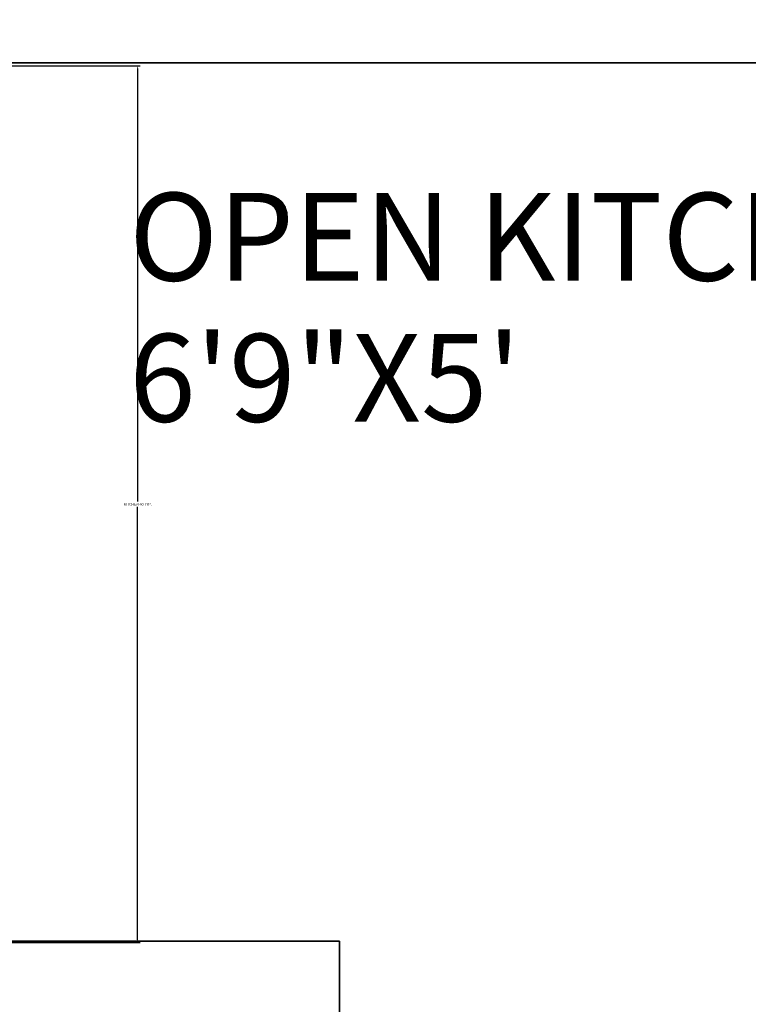
# Model space of a CAD drawing. Units: inches. Extents: x 4159 to 4826, y 299 to 1026.
# Tile 17 of 37: x 4255 to 4305, y 596 to 663. Entities that reach past the tile are written whole.
import ezdxf

# ---------------------------------------------------------------- set-up
doc = ezdxf.new("R2010")
doc.units = ezdxf.units.IN
for name, color, linetype, lineweight in [('A-ANNO-DIMS', 2, 'Continuous', 18), ('A-AREA-IDEN', 7, 'Continuous', 18), ('A-WALL', 7, 'Continuous', 35)]:
    doc.layers.add(name, color=color, linetype=linetype, lineweight=lineweight)
doc.styles.get("Standard").update_dxf_attribs({"font": 'arial.ttf'})
doc.dimstyles.get("Standard").update_dxf_attribs({"dimtxt": 0.18, "dimasz": 0.18, "dimexe": 0.18, "dimexo": 0.0625, "dimgap": 0.09, "dimtad": 0, "dimtih": 1, "dimtoh": 1, "dimdec": 4, "dimzin": 0, "dimdsep": 46, "dimtxsty": 'Standard', "dimcen": 0.09, "dimadec": 0, "dimazin": 0, "dimtfac": 1, "dimtdec": 4, "dimtofl": 0, "dimtmove": 0, "dimatfit": 3, "dimfxl": 1, "dimtolj": 1, "dimtzin": 0, "dimarcsym": 0})

# ---------------------------------------------------------------- blocks, each defined once
blk = doc.blocks.new('*D39')
at = {"layer": 'A-ANNO-DIMS', "color": 0, "lineweight": -2, "transparency": 16777216}
for p, q in [((4254.612, 660.06), (4263.714, 660.06)), ((4263.534, 659.88), (4263.534, 630.296)), ((4263.534, 600.346), (4263.534, 629.93)), ((4254.612, 600.166), (4263.714, 600.166))]:
    blk.add_line(p, q, dxfattribs=at)
at = {"layer": 'A-ANNO-DIMS', "color": 0, "transparency": 16777216}
for points in [[(4263.504, 659.88), (4263.564, 659.88), (4263.534, 660.06)], [(4263.504, 600.346), (4263.564, 600.346), (4263.534, 600.166)]]:
    blk.add_solid(points, dxfattribs=at)
at = {"layer": 'Defpoints', "color": 0, "transparency": 16777216}
for p in [(4254.55, 660.06), (4263.534, 660.06), (4254.55, 600.166)]:
    blk.add_point(p, dxfattribs=at)
at = {"layer": 'A-ANNO-DIMS', "color": 0, "transparency": 16777216, "insert": (4263.534, 630.113), "char_height": 0.18, "attachment_point": 5}
blk.add_mtext('\\A1;KITCHEN 60 TYP.', dxfattribs=at)
blk = doc.blocks.new('*D44')
at = {"layer": 'A-ANNO-DIMS', "color": 0, "lineweight": -2, "transparency": 16777216}
for p, q in [((4287.263, 963.093), (4158.88, 963.093)), ((4159.06, 962.913), (4159.06, 647.826)), ((4159.06, 332.375), (4159.06, 647.462)), ((4447.248, 332.195), (4158.88, 332.195))]:
    blk.add_line(p, q, dxfattribs=at)
at = {"layer": 'A-ANNO-DIMS', "color": 0, "transparency": 16777216}
for points in [[(4159.03, 962.913), (4159.09, 962.913), (4159.06, 963.093)], [(4159.03, 332.375), (4159.09, 332.375), (4159.06, 332.195)]]:
    blk.add_solid(points, dxfattribs=at)
at = {"layer": 'Defpoints', "color": 0, "transparency": 16777216}
for p in [(4287.326, 963.093), (4159.06, 332.195), (4447.31, 332.195)]:
    blk.add_point(p, dxfattribs=at)
at = {"layer": 'A-ANNO-DIMS', "color": 0, "transparency": 16777216, "insert": (4159.06, 647.644), "char_height": 0.18, "attachment_point": 5}
blk.add_mtext('\\A1;630.9', dxfattribs=at)

msp = doc.modelspace()

# ---------------------------------------------------------------- linework, layer by layer
at = {"layer": 'A-WALL'}
for p, q in [((4447.31, 660.254), (4201.31, 660.254)), ((4277.31, 600.254), (4201.31, 600.254)), ((4277.31, 594.254), (4277.31, 600.254))]:
    msp.add_line(p, q, dxfattribs=at)

# ---------------------------------------------------------------- texts
at = {"layer": 'A-AREA-IDEN'}
for s, p in [('OPEN KITCHEN', (4262.954, 645.382)), ('6\'9"X5\'', (4262.954, 635.744))]:
    msp.add_text(s, height=6, dxfattribs=at).set_placement(p)

# ---------------------------------------------------------------- dimensions: what is measured, and where the dimension line sits
at = {"layer": 'A-ANNO-DIMS'}
dim = msp.add_linear_dim(base=(4159.06, 332.195), p1=(4287.326, 963.093), p2=(4447.31, 332.195), angle=90, dimstyle='Standard', override={"dimdec": 1, "dimlfac": 1, "dimrnd": 0, "dimzin": 0, "dimdsep": 46, "dimlunit": 2}, dxfattribs=at)
dim.commit()
dim.dimension.update_dxf_attribs({"geometry": '*D44', "text_midpoint": (4159.06, 647.644)})
dim = msp.add_linear_dim(base=(4263.534, 660.06), p1=(4254.55, 600.166), p2=(4254.55, 660.06), angle=90, text='KITCHEN <> TYP.', dimstyle='Standard', override={"dimdec": 0, "dimlfac": 1, "dimrnd": 0, "dimzin": 0, "dimdsep": 46, "dimlunit": 2}, dxfattribs=at)
dim.commit()
dim.dimension.update_dxf_attribs({"geometry": '*D39', "text_midpoint": (4263.534, 630.113)})

doc.saveas('drawing.dxf')
